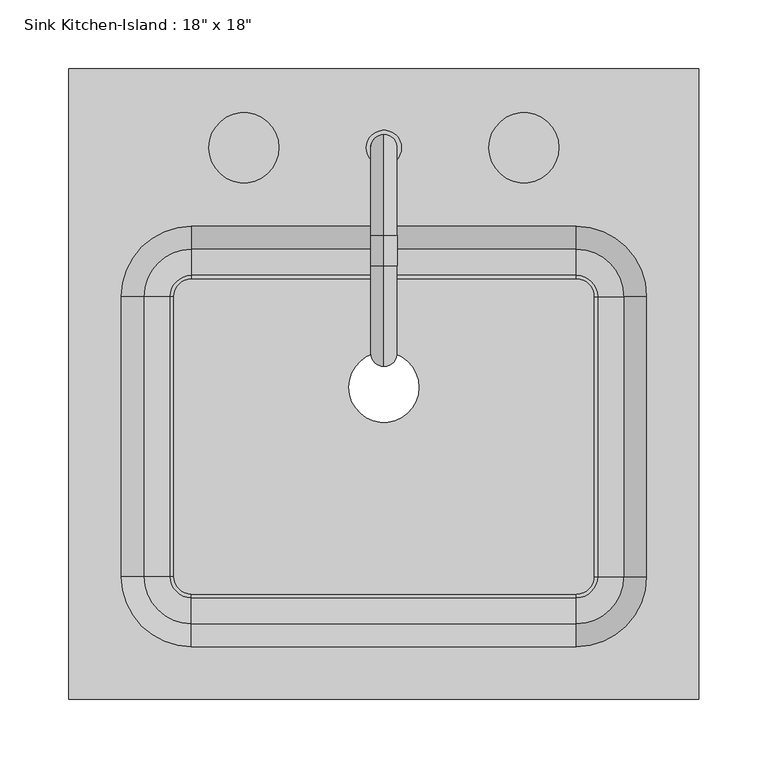
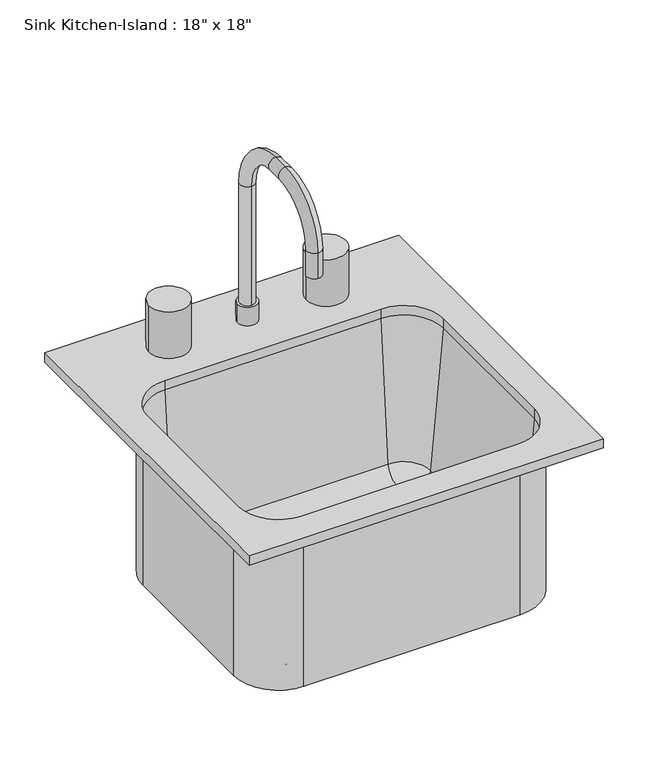
"""IFC4 building model written with IfcOpenShell, lengths in millimetres: flow terminal geometry."""

from ifc_helpers import new_model, si_unit, point, frame, frame_2d, origin, place, context, project, spatial, polyline, circle_curve, ellipse_curve, trimmed, segment, composite_curve, outline, extrude, source, transform, mapped, element, save
from ifc_brep_helpers import plane_surface, cylinder_surface, revolved_surface, advanced_brep


def flow_terminal_2ed30f95(model_context):
    return source(origin(), model_context, "Body", "SolidModel", [
        extrude(outline(composite_curve([segment(trimmed(circle_curve(frame_2d((155.3892406, 65.8454011)), 12.7), [point((155.3892406, 78.5454011))], [point((168.0892406, 65.8454011))], False, "CARTESIAN"), True, "CONTINUOUS"), segment(polyline([(168.0892406, 65.8454011), (168.0892406, -137.3545989)]), True, "CONTINUOUS"), segment(trimmed(circle_curve(frame_2d((155.3892406, -137.3545989)), 12.7), [point((168.0892406, -137.3545989))], [point((155.3892406, -150.0545989))], False, "CARTESIAN"), True, "CONTINUOUS"), segment(polyline([(155.3892406, -150.0545989), (-124.0107594, -150.0545989)]), True, "CONTINUOUS"), segment(trimmed(circle_curve(frame_2d((-124.0107594, -137.3545989)), 12.7), [point((-124.0107594, -150.0545989))], [point((-136.7107594, -137.3545989))], False, "CARTESIAN"), True, "CONTINUOUS"), segment(polyline([(-136.7107594, -137.3545989), (-136.7107594, 65.8454011)]), True, "CONTINUOUS"), segment(trimmed(circle_curve(frame_2d((-124.0107594, 65.8454011)), 12.7), [point((-136.7107594, 65.8454011))], [point((-124.0107594, 78.5454011))], False, "CARTESIAN"), True, "CONTINUOUS"), segment(polyline([(-124.0107594, 78.5454011), (155.3892406, 78.5454011)]), True, "CONTINUOUS")], self_intersect=False), holes=[composite_curve([segment(trimmed(circle_curve(frame_2d((15.6892406, 0.0)), 25.4), [point((-9.7107594, 0.0))], [point((41.0892406, 0.0))], True, "CARTESIAN"), True, "CONTINUOUS"), segment(trimmed(circle_curve(frame_2d((15.6892406, 0.0)), 25.4), [point((41.0892406, 0.0))], [point((-9.7107594, 0.0))], True, "CARTESIAN"), True, "CONTINUOUS")], self_intersect=False)]), frame((0.0, 0.0, 698.5), z_axis=(0.0, 0.0, 1.0), x_axis=(1.0, 0.0, 0.0)), (0.0, 0.0, 1.0), 9.525),
        extrude(outline(composite_curve([segment(trimmed(circle_curve(frame_2d((-85.9107594, 173.7954011)), 25.4), [point((-111.3107594, 173.7954011))], [point((-60.5107594, 173.7954011))], False, "CARTESIAN"), True, "CONTINUOUS"), segment(trimmed(circle_curve(frame_2d((-85.9107594, 173.7954011)), 25.4), [point((-60.5107594, 173.7954011))], [point((-111.3107594, 173.7954011))], False, "CARTESIAN"), True, "CONTINUOUS")], self_intersect=False)), frame((0.0, 0.0, 927.1), z_axis=(0.0, 0.0, 1.0), x_axis=(1.0, 0.0, 0.0)), (0.0, 0.0, 1.0), 63.5),
        extrude(outline(composite_curve([segment(trimmed(circle_curve(frame_2d((117.2892406, 173.7954011)), 25.4), [point((91.8892406, 173.7954011))], [point((142.6892406, 173.7954011))], False, "CARTESIAN"), True, "CONTINUOUS"), segment(trimmed(circle_curve(frame_2d((117.2892406, 173.7954011)), 25.4), [point((142.6892406, 173.7954011))], [point((91.8892406, 173.7954011))], False, "CARTESIAN"), True, "CONTINUOUS")], self_intersect=False)), frame((0.0, 0.0, 927.1), z_axis=(0.0, 0.0, 1.0), x_axis=(1.0, 0.0, 0.0)), (0.0, 0.0, 1.0), 63.5),
        advanced_brep(
        [(2.9892406, 173.7954011, 927.1), (28.3892406, 173.7954011, 927.1), (15.6892406, 183.3204011, 1114.425), (15.6892406, 164.2704011, 1114.425), (15.6892406, 164.2704011, 952.5), (15.6892406, 183.3204011, 952.5), (15.6892406, 110.2954011, 1187.45), (15.6892406, 110.2954011, 1168.4), (15.6892406, 88.0704011, 1187.45), (15.6892406, 88.0704011, 1168.4), (15.6892406, 15.0454011, 1114.425), (15.6892406, 34.0954011, 1114.425), (15.6892406, 15.0454011, 1079.5), (15.6892406, 34.0954011, 1079.5), (2.9892406, 173.7954011, 952.5), (28.3892406, 173.7954011, 952.5)],
        [
            (0, 1, circle_curve(frame((15.6892406, 173.7954011, 927.1), z_axis=(0.0, 0.0, -1.0), x_axis=(1.0, 0.0, 0.0)), 12.7)),
            (1, 0, circle_curve(frame((15.6892406, 173.7954011, 927.1), z_axis=(0.0, 0.0, -1.0), x_axis=(1.0, 0.0, 0.0)), 12.7)),
            (2, 3, circle_curve(frame((15.6892406, 173.7954011, 1114.425), z_axis=(0.0, 0.0, -1.0), x_axis=(0.0, -1.0, 0.0)), 9.525)),
            (3, 4),
            (4, 5, circle_curve(frame((15.6892406, 173.7954011, 952.5), z_axis=(0.0, 0.0, 1.0), x_axis=(0.0, -1.0, 0.0)), 9.525)),
            (5, 2),
            (3, 2, circle_curve(frame((15.6892406, 173.7954011, 1114.425), z_axis=(0.0, 0.0, -1.0), x_axis=(0.0, -1.0, 0.0)), 9.525)),
            (5, 4, circle_curve(frame((15.6892406, 173.7954011, 952.5), z_axis=(0.0, 0.0, 1.0), x_axis=(0.0, -1.0, 0.0)), 9.525)),
            (2, 6, circle_curve(frame((15.6892406, 110.2954011, 1114.425), z_axis=(1.0, 0.0, 0.0), x_axis=(0.0, 1.0, 0.0)), 73.025)),
            (6, 7, circle_curve(frame((15.6892406, 110.2954011, 1177.925), z_axis=(0.0, 1.0, 0.0), x_axis=(0.0, 0.0, -1.0)), 9.525)),
            (7, 3, circle_curve(frame((15.6892406, 110.2954011, 1114.425), z_axis=(-1.0, 0.0, 0.0), x_axis=(0.0, 1.0, 0.0)), 53.975)),
            (7, 6, circle_curve(frame((15.6892406, 110.2954011, 1177.925), z_axis=(0.0, 1.0, 0.0), x_axis=(0.0, 0.0, -1.0)), 9.525)),
            (6, 8),
            (8, 9, circle_curve(frame((15.6892406, 88.0704011, 1177.925), z_axis=(0.0, 1.0, 0.0), x_axis=(0.0, 0.0, -1.0)), 9.525)),
            (9, 7),
            (9, 8, circle_curve(frame((15.6892406, 88.0704011, 1177.925), z_axis=(0.0, 1.0, 0.0), x_axis=(0.0, 0.0, -1.0)), 9.525)),
            (8, 10, circle_curve(frame((15.6892406, 88.0704011, 1114.425), z_axis=(1.0, 0.0, 0.0), x_axis=(0.0, 0.0, 1.0)), 73.025)),
            (10, 11, circle_curve(frame((15.6892406, 24.5704011, 1114.425), z_axis=(0.0, 0.0, 1.0), x_axis=(0.0, 1.0, 0.0)), 9.525)),
            (11, 9, circle_curve(frame((15.6892406, 88.0704011, 1114.425), z_axis=(-1.0, 0.0, 0.0), x_axis=(0.0, 0.0, 1.0)), 53.975)),
            (11, 10, circle_curve(frame((15.6892406, 24.5704011, 1114.425), z_axis=(0.0, 0.0, 1.0), x_axis=(0.0, 1.0, 0.0)), 9.525)),
            (12, 13, circle_curve(frame((15.6892406, 24.5704011, 1079.5), z_axis=(0.0, 0.0, -1.0), x_axis=(0.0, 1.0, 0.0)), 9.525)),
            (13, 12, circle_curve(frame((15.6892406, 24.5704011, 1079.5), z_axis=(0.0, 0.0, -1.0), x_axis=(0.0, 1.0, 0.0)), 9.525)),
            (10, 12),
            (13, 11),
            (14, 15, circle_curve(frame((15.6892406, 173.7954011, 952.5), z_axis=(0.0, 0.0, 1.0), x_axis=(1.0, 0.0, 0.0)), 12.7)),
            (15, 14, circle_curve(frame((15.6892406, 173.7954011, 952.5), z_axis=(0.0, 0.0, 1.0), x_axis=(1.0, 0.0, 0.0)), 12.7)),
            (14, 0),
            (1, 15),
        ],
        [
            plane_surface(frame((15.6892406, 164.2704011, 927.1), z_axis=(0.0, 0.0, -1.0), x_axis=(1.0, 0.0, 0.0))),
            cylinder_surface(frame((15.6892406, 173.7954011, 927.1), z_axis=(0.0, 0.0, -1.0), x_axis=(0.0, -1.0, 0.0)), 9.525),
            revolved_surface(trimmed(ellipse_curve(frame((15.6892406, 173.7954011, 1114.425), z_axis=(0.0, 0.0, -1.0), x_axis=(0.0, -1.0, 0.0)), 9.525, 9.525), [point((15.6892406, 183.3204011, 1114.425))], [point((15.6892406, 164.2704011, 1114.425))], True, "CARTESIAN"), (15.6892406, 110.2954011, 1114.425), (1.0, 0.0, 0.0)),
            revolved_surface(trimmed(ellipse_curve(frame((15.6892406, 173.7954011, 1114.425), z_axis=(0.0, 0.0, -1.0), x_axis=(0.0, -1.0, 0.0)), 9.525, 9.525), [point((15.6892406, 164.2704011, 1114.425))], [point((15.6892406, 183.3204011, 1114.425))], True, "CARTESIAN"), (15.6892406, 110.2954011, 1114.425), (1.0, 0.0, 0.0)),
            cylinder_surface(frame((15.6892406, 110.2954011, 1177.925), z_axis=(0.0, 1.0, 0.0), x_axis=(0.0, 0.0, -1.0)), 9.525),
            revolved_surface(trimmed(ellipse_curve(frame((15.6892406, 88.0704011, 1177.925), z_axis=(0.0, 1.0, 0.0), x_axis=(0.0, 0.0, -1.0)), 9.525, 9.525), [point((15.6892406, 88.0704011, 1187.45))], [point((15.6892406, 88.0704011, 1168.4))], True, "CARTESIAN"), (15.6892406, 88.0704011, 1114.425), (1.0, 0.0, 0.0)),
            revolved_surface(trimmed(ellipse_curve(frame((15.6892406, 88.0704011, 1177.925), z_axis=(0.0, 1.0, 0.0), x_axis=(0.0, 0.0, -1.0)), 9.525, 9.525), [point((15.6892406, 88.0704011, 1168.4))], [point((15.6892406, 88.0704011, 1187.45))], True, "CARTESIAN"), (15.6892406, 88.0704011, 1114.425), (1.0, 0.0, 0.0)),
            plane_surface(frame((15.6892406, 15.0454011, 1079.5), z_axis=(0.0, 0.0, -1.0), x_axis=(-1.0, 0.0, 0.0))),
            cylinder_surface(frame((15.6892406, 24.5704011, 1114.425), z_axis=(0.0, 0.0, 1.0), x_axis=(0.0, 1.0, 0.0)), 9.525),
            plane_surface(frame((28.3892406, 173.7954011, 952.5), z_axis=(0.0, 0.0, 1.0), x_axis=(0.0, 1.0, 0.0))),
            cylinder_surface(frame((15.6892406, 173.7954011, 927.1), z_axis=(0.0, 0.0, 1.0), x_axis=(1.0, 0.0, 0.0)), 12.7),
        ],
        [
            (0, [[1, 2]]),
            (1, [[3, 4, 5, 6]]),
            (1, [[7, -6, 8, -4]]),
            (2, [[-3, 9, 10, 11]]),
            (3, [[-7, -11, 12, -9]]),
            (4, [[-10, 13, 14, 15]]),
            (4, [[-12, -15, 16, -13]]),
            (5, [[-14, 17, 18, 19]]),
            (6, [[-16, -19, 20, -17]]),
            (7, [[21, 22]]),
            (8, [[-18, 23, -22, 24]]),
            (8, [[-20, -24, -21, -23]]),
            (9, [[25, 26], [-5, -8]]),
            (10, [[-25, 27, -2, 28]]),
            (10, [[-26, -28, -1, -27]]),
        ],
    ),
        advanced_brep(
        [(244.2892406, 230.9454011, 927.1), (-212.9107594, 230.9454011, 927.1), (-212.9107594, -226.2545989, 927.1), (244.2892406, -226.2545989, 927.1), (155.3892406, 116.6454011, 927.1), (206.1892406, 65.8454011, 927.1), (206.1892406, -137.3545989, 927.1), (155.3892406, -188.1545989, 927.1), (-124.0107594, -188.1545989, 927.1), (-174.8107594, -137.3545989, 927.1), (-174.8107594, 65.8454011, 927.1), (-124.0107594, 116.6454011, 927.1), (244.2892406, 230.9454011, 914.4), (244.2892406, -226.2545989, 914.4), (-212.9107594, -226.2545989, 914.4), (-212.9107594, 230.9454011, 914.4), (212.5392406, 65.8454011, 914.4), (155.3892406, 122.9954011, 914.4), (-124.0107594, 122.9954011, 914.4), (-181.1607594, 65.8454011, 914.4), (-181.1607594, -137.3545989, 914.4), (-124.0107594, -194.5045989, 914.4), (155.3892406, -194.5045989, 914.4), (212.5392406, -137.3545989, 914.4), (155.3892406, 116.6454011, 914.4), (206.1892406, 65.8454011, 914.4), (206.1892406, -137.3545989, 914.4), (155.3892406, -188.1545989, 914.4), (-124.0107594, -188.1545989, 914.4), (-174.8107594, -137.3545989, 914.4), (-174.8107594, 65.8454011, 914.4), (-124.0107594, 116.6454011, 914.4), (212.5392406, 65.8454011, 698.5), (155.3892406, 122.9954011, 698.5), (168.0892406, 65.8454011, 698.5), (155.3892406, 78.5454011, 698.5), (168.0892406, 65.8454011, 708.025), (155.3892406, 78.5454011, 708.025), (170.6776588, 65.8454011, 708.025), (155.3892406, 81.1338193, 708.025), (189.6551678, 65.8454011, 725.4146831), (155.3892406, 100.1113283, 725.4146831), (212.5392406, -137.3545989, 698.5), (168.0892406, -137.3545989, 698.5), (168.0892406, -137.3545989, 708.025), (170.6776588, -137.3545989, 708.025), (189.6551678, -137.3545989, 725.4146831), (155.3892406, -194.5045989, 698.5), (155.3892406, -150.0545989, 698.5), (155.3892406, -150.0545989, 708.025), (155.3892406, -152.6430171, 708.025), (155.3892406, -171.6205261, 725.4146831), (-124.0107594, -194.5045989, 698.5), (-124.0107594, -150.0545989, 698.5), (-124.0107594, -150.0545989, 708.025), (-124.0107594, -152.6430171, 708.025), (-124.0107594, -171.6205261, 725.4146831), (-181.1607594, -137.3545989, 698.5), (-136.7107594, -137.3545989, 698.5), (-136.7107594, -137.3545989, 708.025), (-139.2991776, -137.3545989, 708.025), (-158.2766866, -137.3545989, 725.4146831), (-181.1607594, 65.8454011, 698.5), (-136.7107594, 65.8454011, 698.5), (-136.7107594, 65.8454011, 708.025), (-139.2991776, 65.8454011, 708.025), (-158.2766866, 65.8454011, 725.4146831), (-124.0107594, 122.9954011, 698.5), (-124.0107594, 78.5454011, 698.5), (-124.0107594, 78.5454011, 708.025), (-124.0107594, 81.1338193, 708.025), (-124.0107594, 100.1113283, 725.4146831)],
        [
            (0, 1),
            (1, 2),
            (2, 3),
            (3, 0),
            (4, 5, circle_curve(frame((155.3892406, 65.8454011, 927.1), z_axis=(0.0, 0.0, -1.0), x_axis=(1.0, 0.0, 0.0)), 50.8)),
            (5, 6),
            (6, 7, circle_curve(frame((155.3892406, -137.3545989, 927.1), z_axis=(0.0, 0.0, -1.0), x_axis=(1.0, 0.0, 0.0)), 50.8)),
            (7, 8),
            (8, 9, circle_curve(frame((-124.0107594, -137.3545989, 927.1), z_axis=(0.0, 0.0, -1.0), x_axis=(1.0, 0.0, 0.0)), 50.8)),
            (9, 10),
            (10, 11, circle_curve(frame((-124.0107594, 65.8454011, 927.1), z_axis=(0.0, 0.0, -1.0), x_axis=(1.0, 0.0, 0.0)), 50.8)),
            (11, 4),
            (12, 13),
            (13, 14),
            (14, 15),
            (15, 12),
            (16, 17, circle_curve(frame((155.3892406, 65.8454011, 914.4), z_axis=(0.0, 0.0, 1.0), x_axis=(0.0, 1.0, 0.0)), 57.15)),
            (17, 18),
            (18, 19, circle_curve(frame((-124.0107594, 65.8454011, 914.4), z_axis=(0.0, 0.0, 1.0), x_axis=(-1.0, 0.0, 0.0)), 57.15)),
            (19, 20),
            (20, 21, circle_curve(frame((-124.0107594, -137.3545989, 914.4), z_axis=(0.0, 0.0, 1.0), x_axis=(0.0, -1.0, 0.0)), 57.15)),
            (21, 22),
            (22, 23, circle_curve(frame((155.3892406, -137.3545989, 914.4), z_axis=(0.0, 0.0, 1.0), x_axis=(1.0, 0.0, 0.0)), 57.15)),
            (23, 16),
            (0, 12),
            (15, 1),
            (14, 2),
            (13, 3),
            (4, 24),
            (24, 25, circle_curve(frame((155.3892406, 65.8454011, 914.4), z_axis=(0.0, 0.0, -1.0), x_axis=(1.0, 0.0, 0.0)), 50.8)),
            (25, 5),
            (25, 26),
            (26, 6),
            (26, 27, circle_curve(frame((155.3892406, -137.3545989, 914.4), z_axis=(0.0, 0.0, -1.0), x_axis=(1.0, 0.0, 0.0)), 50.8)),
            (27, 7),
            (27, 28),
            (28, 8),
            (28, 29, circle_curve(frame((-124.0107594, -137.3545989, 914.4), z_axis=(0.0, 0.0, -1.0), x_axis=(1.0, 0.0, 0.0)), 50.8)),
            (29, 9),
            (29, 30),
            (30, 10),
            (30, 31, circle_curve(frame((-124.0107594, 65.8454011, 914.4), z_axis=(0.0, 0.0, -1.0), x_axis=(1.0, 0.0, 0.0)), 50.8)),
            (31, 11),
            (31, 24),
            (32, 33, circle_curve(frame((155.3892406, 65.8454011, 698.5), z_axis=(0.0, 0.0, 1.0), x_axis=(0.0, 1.0, 0.0)), 57.15)),
            (33, 17),
            (16, 32),
            (32, 34),
            (34, 35, circle_curve(frame((155.3892406, 65.8454011, 698.5), z_axis=(0.0, 0.0, 1.0), x_axis=(0.0, 1.0, 0.0)), 12.7)),
            (35, 33),
            (34, 36),
            (36, 37, circle_curve(frame((155.3892406, 65.8454011, 708.025), z_axis=(0.0, 0.0, 1.0), x_axis=(0.0, 1.0, 0.0)), 12.7)),
            (37, 35),
            (36, 38),
            (38, 39, circle_curve(frame((155.3892406, 65.8454011, 708.025), z_axis=(0.0, 0.0, 1.0), x_axis=(0.0, 1.0, 0.0)), 15.2884182)),
            (39, 37),
            (38, 40, circle_curve(frame((170.6776588, 65.8454011, 727.075), z_axis=(0.0, -1.0, 0.0), x_axis=(1.0, 0.0, 0.0)), 19.05)),
            (40, 41, circle_curve(frame((155.3892406, 65.8454011, 725.4146831), z_axis=(0.0, 0.0, 1.0), x_axis=(0.0, 1.0, 0.0)), 34.2659272)),
            (41, 39, circle_curve(frame((155.3892406, 81.1338193, 727.075), z_axis=(-1.0, 0.0, 0.0), x_axis=(0.0, 1.0, 0.0)), 19.05)),
            (40, 25),
            (24, 41),
            (23, 42),
            (42, 32),
            (42, 43),
            (43, 34),
            (43, 44),
            (44, 36),
            (44, 45),
            (45, 38),
            (45, 46, circle_curve(frame((170.6776588, -137.3545989, 727.075), z_axis=(0.0, -1.0, 0.0), x_axis=(1.0, 0.0, 0.0)), 19.05)),
            (46, 40),
            (46, 26),
            (22, 47),
            (47, 42, circle_curve(frame((155.3892406, -137.3545989, 698.5), z_axis=(0.0, 0.0, 1.0), x_axis=(1.0, 0.0, 0.0)), 57.15)),
            (47, 48),
            (48, 43, circle_curve(frame((155.3892406, -137.3545989, 698.5), z_axis=(0.0, 0.0, 1.0), x_axis=(1.0, 0.0, 0.0)), 12.7)),
            (48, 49),
            (49, 44, circle_curve(frame((155.3892406, -137.3545989, 708.025), z_axis=(0.0, 0.0, 1.0), x_axis=(1.0, 0.0, 0.0)), 12.7)),
            (49, 50),
            (50, 45, circle_curve(frame((155.3892406, -137.3545989, 708.025), z_axis=(0.0, 0.0, 1.0), x_axis=(1.0, 0.0, 0.0)), 15.2884182)),
            (50, 51, circle_curve(frame((155.3892406, -152.6430171, 727.075), z_axis=(-1.0, 0.0, 0.0), x_axis=(0.0, -1.0, 0.0)), 19.05)),
            (51, 46, circle_curve(frame((155.3892406, -137.3545989, 725.4146831), z_axis=(0.0, 0.0, 1.0), x_axis=(1.0, 0.0, 0.0)), 34.2659272)),
            (51, 27),
            (21, 52),
            (52, 47),
            (52, 53),
            (53, 48),
            (53, 54),
            (54, 49),
            (54, 55),
            (55, 50),
            (55, 56, circle_curve(frame((-124.0107594, -152.6430171, 727.075), z_axis=(-1.0, 0.0, 0.0), x_axis=(0.0, -1.0, 0.0)), 19.05)),
            (56, 51),
            (56, 28),
            (20, 57),
            (57, 52, circle_curve(frame((-124.0107594, -137.3545989, 698.5), z_axis=(0.0, 0.0, 1.0), x_axis=(0.0, -1.0, 0.0)), 57.15)),
            (57, 58),
            (58, 53, circle_curve(frame((-124.0107594, -137.3545989, 698.5), z_axis=(0.0, 0.0, 1.0), x_axis=(0.0, -1.0, 0.0)), 12.7)),
            (58, 59),
            (59, 54, circle_curve(frame((-124.0107594, -137.3545989, 708.025), z_axis=(0.0, 0.0, 1.0), x_axis=(0.0, -1.0, 0.0)), 12.7)),
            (59, 60),
            (60, 55, circle_curve(frame((-124.0107594, -137.3545989, 708.025), z_axis=(0.0, 0.0, 1.0), x_axis=(0.0, -1.0, 0.0)), 15.2884182)),
            (60, 61, circle_curve(frame((-139.2991776, -137.3545989, 727.075), z_axis=(0.0, 1.0, 0.0), x_axis=(-1.0, 0.0, 0.0)), 19.05)),
            (61, 56, circle_curve(frame((-124.0107594, -137.3545989, 725.4146831), z_axis=(0.0, 0.0, 1.0), x_axis=(0.0, -1.0, 0.0)), 34.2659272)),
            (61, 29),
            (19, 62),
            (62, 57),
            (62, 63),
            (63, 58),
            (63, 64),
            (64, 59),
            (64, 65),
            (65, 60),
            (65, 66, circle_curve(frame((-139.2991776, 65.8454011, 727.075), z_axis=(0.0, 1.0, 0.0), x_axis=(-1.0, 0.0, 0.0)), 19.05)),
            (66, 61),
            (66, 30),
            (18, 67),
            (67, 62, circle_curve(frame((-124.0107594, 65.8454011, 698.5), z_axis=(0.0, 0.0, 1.0), x_axis=(-1.0, 0.0, 0.0)), 57.15)),
            (67, 68),
            (68, 63, circle_curve(frame((-124.0107594, 65.8454011, 698.5), z_axis=(0.0, 0.0, 1.0), x_axis=(-1.0, 0.0, 0.0)), 12.7)),
            (68, 69),
            (69, 64, circle_curve(frame((-124.0107594, 65.8454011, 708.025), z_axis=(0.0, 0.0, 1.0), x_axis=(-1.0, 0.0, 0.0)), 12.7)),
            (69, 70),
            (70, 65, circle_curve(frame((-124.0107594, 65.8454011, 708.025), z_axis=(0.0, 0.0, 1.0), x_axis=(-1.0, 0.0, 0.0)), 15.2884182)),
            (70, 71, circle_curve(frame((-124.0107594, 81.1338193, 727.075), z_axis=(1.0, 0.0, 0.0), x_axis=(0.0, 1.0, 0.0)), 19.05)),
            (71, 66, circle_curve(frame((-124.0107594, 65.8454011, 725.4146831), z_axis=(0.0, 0.0, 1.0), x_axis=(-1.0, 0.0, 0.0)), 34.2659272)),
            (71, 31),
            (33, 67),
            (35, 68),
            (37, 69),
            (39, 70),
            (41, 71),
        ],
        [
            plane_surface(frame((-212.9107594, 230.9454011, 927.1), z_axis=(0.0, 0.0, 1.0), x_axis=(-1.0, 0.0, 0.0))),
            plane_surface(frame((-212.9107594, 230.9454011, 914.4), z_axis=(0.0, 0.0, -1.0), x_axis=(1.0, 0.0, 0.0))),
            plane_surface(frame((244.2892406, 230.9454011, 927.1), z_axis=(0.0, 1.0, 0.0), x_axis=(0.0, 0.0, -1.0))),
            plane_surface(frame((-212.9107594, 230.9454011, 927.1), z_axis=(-1.0, 0.0, 0.0), x_axis=(0.0, 0.0, -1.0))),
            plane_surface(frame((-212.9107594, -226.2545989, 927.1), z_axis=(0.0, -1.0, 0.0), x_axis=(0.0, 0.0, -1.0))),
            plane_surface(frame((244.2892406, -226.2545989, 927.1), z_axis=(1.0, 0.0, 0.0), x_axis=(0.0, 0.0, -1.0))),
            revolved_surface(polyline([(206.1892406, 65.8454011, 914.4), (206.1892406, 65.8454011, 927.1)]), (155.3892406, 65.8454011, 0.0), (0.0, 0.0, -1.0)),
            plane_surface(frame((206.1892406, 65.8454011, 927.1), z_axis=(-1.0, 0.0, 0.0), x_axis=(0.0, 0.0, -1.0))),
            revolved_surface(polyline([(206.1892406, -137.3545989, 914.4), (206.1892406, -137.3545989, 927.1)]), (155.3892406, -137.3545989, 0.0), (0.0, 0.0, -1.0)),
            plane_surface(frame((155.3892406, -188.1545989, 927.1), z_axis=(0.0, 1.0, 0.0), x_axis=(0.0, 0.0, -1.0))),
            revolved_surface(polyline([(-73.2107594, -137.3545989, 914.4), (-73.2107594, -137.3545989, 927.1)]), (-124.0107594, -137.3545989, 0.0), (0.0, 0.0, -1.0)),
            plane_surface(frame((-174.8107594, -137.3545989, 927.1), z_axis=(1.0, 0.0, 0.0), x_axis=(0.0, 0.0, -1.0))),
            revolved_surface(polyline([(-73.2107594, 65.8454011, 914.4), (-73.2107594, 65.8454011, 927.1)]), (-124.0107594, 65.8454011, 0.0), (0.0, 0.0, -1.0)),
            plane_surface(frame((-124.0107594, 116.6454011, 927.1), z_axis=(0.0, -1.0, 0.0), x_axis=(0.0, 0.0, -1.0))),
            cylinder_surface(frame((155.3892406, 65.8454011, 0.0), z_axis=(0.0, 0.0, -1.0), x_axis=(0.0, 1.0, 0.0)), 57.15),
            plane_surface(frame((155.3892406, 65.8454011, 698.5), z_axis=(0.0, 0.0, -1.0), x_axis=(0.0, 1.0, 0.0))),
            revolved_surface(polyline([(155.3892406, 78.5454011, 698.5), (155.3892406, 78.5454011, 708.025)]), (155.3892406, 65.8454011, 0.0), (0.0, 0.0, -1.0)),
            plane_surface(frame((155.3892406, 65.8454011, 708.025), z_axis=(0.0, 0.0, 1.0), x_axis=(0.0, 1.0, 0.0))),
            revolved_surface(trimmed(ellipse_curve(frame((155.3892406, 81.1338193, 727.075), z_axis=(1.0, 0.0, 0.0), x_axis=(0.0, 1.0, 0.0)), 19.05, 19.05), [point((155.3892406, 81.1338193, 708.025))], [point((155.3892406, 100.1113283, 725.4146831))], True, "CARTESIAN"), (155.3892406, 65.8454011, 0.0), (0.0, 0.0, -1.0)),
            revolved_surface(polyline([(155.3892406, 100.1113283, 725.4146831), (155.3892406, 116.6454011, 914.4)]), (155.3892406, 65.8454011, 0.0), (0.0, 0.0, -1.0)),
            plane_surface(frame((212.5392406, 65.8454011, 914.4), z_axis=(1.0, 0.0, 0.0), x_axis=(0.0, -1.0, 0.0))),
            plane_surface(frame((212.5392406, 65.8454011, 698.5), z_axis=(0.0, 0.0, -1.0), x_axis=(0.0, -1.0, 0.0))),
            plane_surface(frame((168.0892406, 65.8454011, 698.5), z_axis=(-1.0, 0.0, 0.0), x_axis=(0.0, -1.0, 0.0))),
            plane_surface(frame((168.0892406, 65.8454011, 708.025), z_axis=(0.0, 0.0, 1.0), x_axis=(0.0, -1.0, 0.0))),
            revolved_surface(polyline([(189.7276588, -137.3545989, 727.075), (189.7276588, 65.8454011, 727.075)]), (170.6776588, 65.8454011, 727.075), (0.0, -1.0, 0.0)),
            plane_surface(frame((189.6551678, 65.8454011, 725.4146831), z_axis=(-0.9961946980917443, 0.0, 0.08715574274767254), x_axis=(0.0, -1.0, 0.0))),
            cylinder_surface(frame((155.3892406, -137.3545989, 0.0), z_axis=(0.0, 0.0, -1.0), x_axis=(1.0, 0.0, 0.0)), 57.15),
            plane_surface(frame((155.3892406, -137.3545989, 698.5), z_axis=(0.0, 0.0, -1.0), x_axis=(1.0, 0.0, 0.0))),
            revolved_surface(polyline([(168.08924059999998, -137.3545989, 698.5), (168.08924059999998, -137.3545989, 708.025)]), (155.3892406, -137.3545989, 0.0), (0.0, 0.0, -1.0)),
            plane_surface(frame((155.3892406, -137.3545989, 708.025), z_axis=(0.0, 0.0, 1.0), x_axis=(1.0, 0.0, 0.0))),
            revolved_surface(trimmed(ellipse_curve(frame((170.6776588, -137.3545989, 727.075), z_axis=(0.0, -1.0, 0.0), x_axis=(1.0, 0.0, 0.0)), 19.05, 19.05), [point((170.6776588, -137.3545989, 708.025))], [point((189.6551678, -137.3545989, 725.4146831))], True, "CARTESIAN"), (155.3892406, -137.3545989, 0.0), (0.0, 0.0, -1.0)),
            revolved_surface(polyline([(189.6551678, -137.3545989, 725.4146831), (206.1892406, -137.3545989, 914.4)]), (155.3892406, -137.3545989, 0.0), (0.0, 0.0, -1.0)),
            plane_surface(frame((155.3892406, -194.5045989, 914.4), z_axis=(0.0, -1.0, 0.0), x_axis=(-1.0, 0.0, 0.0))),
            plane_surface(frame((155.3892406, -194.5045989, 698.5), z_axis=(0.0, 0.0, -1.0), x_axis=(-1.0, 0.0, 0.0))),
            plane_surface(frame((155.3892406, -150.0545989, 698.5), z_axis=(0.0, 1.0, 0.0), x_axis=(-1.0, 0.0, 0.0))),
            plane_surface(frame((155.3892406, -150.0545989, 708.025), z_axis=(0.0, 0.0, 1.0), x_axis=(-1.0, 0.0, 0.0))),
            revolved_surface(polyline([(-124.01075939999998, -171.69301710000002, 727.075), (155.3892406, -171.69301710000002, 727.075)]), (155.3892406, -152.6430171, 727.075), (-1.0, 0.0, 0.0)),
            plane_surface(frame((155.3892406, -171.6205261, 725.4146831), z_axis=(0.0, 0.9961946980917443, 0.08715574274767254), x_axis=(-1.0, 0.0, 0.0))),
            cylinder_surface(frame((-124.0107594, -137.3545989, 0.0), z_axis=(0.0, 0.0, -1.0), x_axis=(0.0, -1.0, 0.0)), 57.15),
            plane_surface(frame((-124.0107594, -137.3545989, 698.5), z_axis=(0.0, 0.0, -1.0), x_axis=(0.0, -1.0, 0.0))),
            revolved_surface(polyline([(-124.0107594, -150.0545989, 698.5), (-124.0107594, -150.0545989, 708.025)]), (-124.0107594, -137.3545989, 0.0), (0.0, 0.0, -1.0)),
            plane_surface(frame((-124.0107594, -137.3545989, 708.025), z_axis=(0.0, 0.0, 1.0), x_axis=(0.0, -1.0, 0.0))),
            revolved_surface(trimmed(ellipse_curve(frame((-124.0107594, -152.6430171, 727.075), z_axis=(-1.0, 0.0, 0.0), x_axis=(0.0, -1.0, 0.0)), 19.05, 19.05), [point((-124.0107594, -152.6430171, 708.025))], [point((-124.0107594, -171.6205261, 725.4146831))], True, "CARTESIAN"), (-124.0107594, -137.3545989, 0.0), (0.0, 0.0, -1.0)),
            revolved_surface(polyline([(-124.0107594, -171.6205261, 725.4146831), (-124.0107594, -188.1545989, 914.4)]), (-124.0107594, -137.3545989, 0.0), (0.0, 0.0, -1.0)),
            plane_surface(frame((-181.1607594, -137.3545989, 914.4), z_axis=(-1.0, 0.0, 0.0), x_axis=(0.0, 1.0, 0.0))),
            plane_surface(frame((-181.1607594, -137.3545989, 698.5), z_axis=(0.0, 0.0, -1.0), x_axis=(0.0, 1.0, 0.0))),
            plane_surface(frame((-136.7107594, -137.3545989, 698.5), z_axis=(1.0, 0.0, 0.0), x_axis=(0.0, 1.0, 0.0))),
            plane_surface(frame((-136.7107594, -137.3545989, 708.025), z_axis=(0.0, 0.0, 1.0), x_axis=(0.0, 1.0, 0.0))),
            revolved_surface(polyline([(-158.34917760000002, 65.8454011, 727.075), (-158.34917760000002, -137.3545989, 727.075)]), (-139.2991776, -137.3545989, 727.075), (0.0, 1.0, 0.0)),
            plane_surface(frame((-158.2766866, -137.3545989, 725.4146831), z_axis=(0.9961946980917443, 0.0, 0.08715574274767254), x_axis=(0.0, 1.0, 0.0))),
            cylinder_surface(frame((-124.0107594, 65.8454011, 0.0), z_axis=(0.0, 0.0, -1.0), x_axis=(-1.0, 0.0, 0.0)), 57.15),
            plane_surface(frame((-124.0107594, 65.8454011, 698.5), z_axis=(0.0, 0.0, -1.0), x_axis=(-1.0, 0.0, 0.0))),
            revolved_surface(polyline([(-136.7107594, 65.8454011, 698.5), (-136.7107594, 65.8454011, 708.025)]), (-124.0107594, 65.8454011, 0.0), (0.0, 0.0, -1.0)),
            plane_surface(frame((-124.0107594, 65.8454011, 708.025), z_axis=(0.0, 0.0, 1.0), x_axis=(-1.0, 0.0, 0.0))),
            revolved_surface(trimmed(ellipse_curve(frame((-139.2991776, 65.8454011, 727.075), z_axis=(0.0, 1.0, 0.0), x_axis=(-1.0, 0.0, 0.0)), 19.05, 19.05), [point((-139.2991776, 65.8454011, 708.025))], [point((-158.2766866, 65.8454011, 725.4146831))], True, "CARTESIAN"), (-124.0107594, 65.8454011, 0.0), (0.0, 0.0, -1.0)),
            revolved_surface(polyline([(-158.2766866, 65.8454011, 725.4146831), (-174.8107594, 65.8454011, 914.4)]), (-124.0107594, 65.8454011, 0.0), (0.0, 0.0, -1.0)),
            plane_surface(frame((-124.0107594, 122.9954011, 914.4), z_axis=(0.0, 1.0, 0.0), x_axis=(1.0, 0.0, 0.0))),
            plane_surface(frame((-124.0107594, 122.9954011, 698.5), z_axis=(0.0, 0.0, -1.0), x_axis=(1.0, 0.0, 0.0))),
            plane_surface(frame((-124.0107594, 78.5454011, 698.5), z_axis=(0.0, -1.0, 0.0), x_axis=(1.0, 0.0, 0.0))),
            plane_surface(frame((-124.0107594, 78.5454011, 708.025), z_axis=(0.0, 0.0, 1.0), x_axis=(1.0, 0.0, 0.0))),
            revolved_surface(polyline([(155.3892406, 100.1838193, 727.075), (-124.0107594, 100.1838193, 727.075)]), (-124.0107594, 81.1338193, 727.075), (1.0, 0.0, 0.0)),
            plane_surface(frame((-124.0107594, 100.1113283, 725.4146831), z_axis=(0.0, -0.9961946980917443, 0.08715574274767254), x_axis=(1.0, 0.0, 0.0))),
        ],
        [
            (0, [[1, 2, 3, 4], [5, 6, 7, 8, 9, 10, 11, 12]]),
            (1, [[13, 14, 15, 16], [17, 18, 19, 20, 21, 22, 23, 24]]),
            (2, [[-1, 25, -16, 26]]),
            (3, [[-2, -26, -15, 27]]),
            (4, [[-3, -27, -14, 28]]),
            (5, [[-4, -28, -13, -25]]),
            (6, [[-5, 29, 30, 31]]),
            (7, [[-6, -31, 32, 33]]),
            (8, [[-7, -33, 34, 35]]),
            (9, [[-8, -35, 36, 37]]),
            (10, [[-9, -37, 38, 39]]),
            (11, [[-10, -39, 40, 41]]),
            (12, [[-11, -41, 42, 43]]),
            (13, [[-12, -43, 44, -29]]),
            (14, [[45, 46, -17, 47]]),
            (15, [[-45, 48, 49, 50]]),
            (16, [[-49, 51, 52, 53]]),
            (17, [[-52, 54, 55, 56]]),
            (18, [[-55, 57, 58, 59]]),
            (19, [[-58, 60, -30, 61]]),
            (20, [[-47, -24, 62, 63]]),
            (21, [[-48, -63, 64, 65]]),
            (22, [[-51, -65, 66, 67]]),
            (23, [[-54, -67, 68, 69]]),
            (24, [[-57, -69, 70, 71]]),
            (25, [[-60, -71, 72, -32]]),
            (26, [[-62, -23, 73, 74]]),
            (27, [[-64, -74, 75, 76]]),
            (28, [[-66, -76, 77, 78]]),
            (29, [[-68, -78, 79, 80]]),
            (30, [[-70, -80, 81, 82]]),
            (31, [[-72, -82, 83, -34]]),
            (32, [[-73, -22, 84, 85]]),
            (33, [[-75, -85, 86, 87]]),
            (34, [[-77, -87, 88, 89]]),
            (35, [[-79, -89, 90, 91]]),
            (36, [[-81, -91, 92, 93]]),
            (37, [[-83, -93, 94, -36]]),
            (38, [[-84, -21, 95, 96]]),
            (39, [[-86, -96, 97, 98]]),
            (40, [[-88, -98, 99, 100]]),
            (41, [[-90, -100, 101, 102]]),
            (42, [[-92, -102, 103, 104]]),
            (43, [[-94, -104, 105, -38]]),
            (44, [[-95, -20, 106, 107]]),
            (45, [[-97, -107, 108, 109]]),
            (46, [[-99, -109, 110, 111]]),
            (47, [[-101, -111, 112, 113]]),
            (48, [[-103, -113, 114, 115]]),
            (49, [[-105, -115, 116, -40]]),
            (50, [[-106, -19, 117, 118]]),
            (51, [[-108, -118, 119, 120]]),
            (52, [[-110, -120, 121, 122]]),
            (53, [[-112, -122, 123, 124]]),
            (54, [[-114, -124, 125, 126]]),
            (55, [[-116, -126, 127, -42]]),
            (56, [[-46, 128, -117, -18]]),
            (57, [[-50, 129, -119, -128]]),
            (58, [[-53, 130, -121, -129]]),
            (59, [[-56, 131, -123, -130]]),
            (60, [[-59, 132, -125, -131]]),
            (61, [[-61, -44, -127, -132]]),
        ],
    ),
    ])


if __name__ == "__main__":
    model = new_model("IFC4")
    model_context = context("Model", 3, world=origin())
    ifc_project = project(units=[si_unit("LENGTHUNIT", "METRE", prefix="MILLI")], contexts=[model_context])
    site = spatial("IfcSite", under=ifc_project)
    building = spatial("IfcBuilding", under=site)
    placement = place(None, origin())
    flow_terminal_shape = flow_terminal_2ed30f95(model_context)
    element("IfcFlowTerminal", 1, ObjectType="Sink Kitchen-Island : 18\" x 18\"", at=placement, inside=building, context=model_context, shape_type="MappedRepresentation", body=[
        mapped(flow_terminal_shape, transform((0.0, 0.0, 0.0), x_axis=(1.0, 0.0, 0.0), y_axis=(0.0, 1.0, 0.0), z_axis=(0.0, 0.0, 1.0))),
    ])
    save(model, "model.ifc")

# Revit data of these elements
# Type "Sink Kitchen-Island : 18\" x 18\""
#   Assembly Code = "D2010410"
#   Counter Height = 3' - 0"
#   Depth = 1' - 6"
#   Width = 1' - 6"
#   Faucet Material = Steel, Polished
#   Sink Material = Steel, Polished
#   Default Elevation = 0
# Element 1 (IfcFlowTerminal, "Sink Kitchen-Island : 18\" x 18\"")
#   Materials on its faces: "Steel, Polished"
# Materials
#   "Steel, Polished": class "Metal", colour RGB 57 57 57, transparency 0, Description = "Polished steel", Cost = 0
